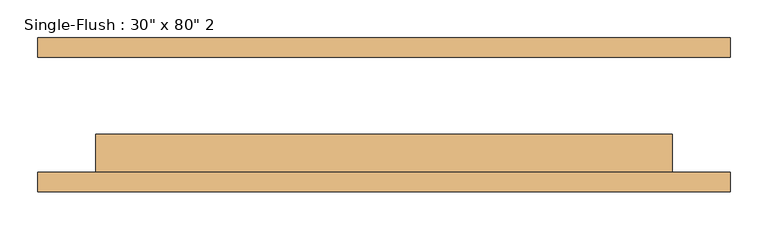
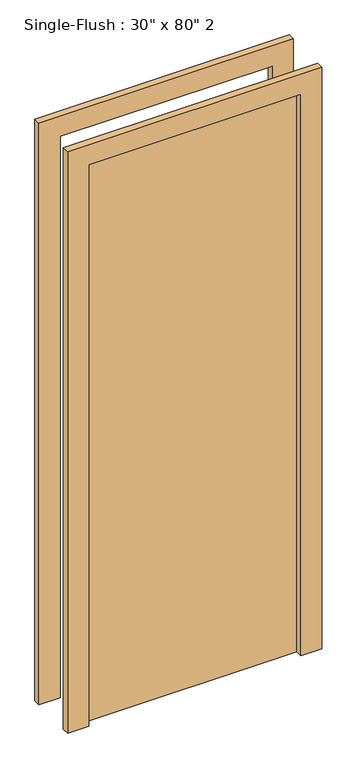
"""IFC4 building model written with IfcOpenShell, lengths in millimetres: door geometry."""

from ifc_helpers import new_model, si_unit, frame, origin, origin_with_axes, place, context, project, spatial, polyline, outline, extrude, source, transform, mapped, element, save


def door_e2b13fe9(model_context):
    return source(origin(), model_context, "Body", "SweptSolid", [
        extrude(outline(polyline([(2209.8, -457.2), (0.0, -457.2), (0.0, -381.0), (2133.6, -381.0), (2133.6, 381.0), (0.0, 381.0), (0.0, 457.2), (2209.8, 457.2), (2209.8, -457.2)])), frame((0.0, -101.6, 0.0), z_axis=(0.0, 1.0, 0.0), x_axis=(0.0, 0.0, 1.0)), (0.0, 0.0, 1.0), 25.4),
        extrude(outline(polyline([(2209.8, 457.2), (2209.8, -457.2), (0.0, -457.2), (0.0, -381.0), (2133.6, -381.0), (2133.6, 381.0), (0.0, 381.0), (0.0, 457.2), (2209.8, 457.2)])), frame((0.0, 76.2, 0.0), z_axis=(0.0, 1.0, 0.0), x_axis=(0.0, 0.0, 1.0)), (0.0, 0.0, 1.0), 25.4),
        extrude(outline(polyline([(381.0, -25.4), (381.0, -76.2), (-381.0, -76.2), (-381.0, -25.4), (381.0, -25.4)])), origin_with_axes(), (0.0, 0.0, 1.0), 2133.6),
    ])


if __name__ == "__main__":
    model = new_model("IFC4")
    model_context = context("Model", 3, world=origin())
    ifc_project = project(units=[si_unit("LENGTHUNIT", "METRE", prefix="MILLI")], contexts=[model_context])
    site = spatial("IfcSite", under=ifc_project)
    building = spatial("IfcBuilding", under=site)
    placement = place(None, origin())
    door_shape = door_e2b13fe9(model_context)
    element("IfcDoor", 1, ObjectType="Single-Flush : 30\" x 80\" 2", at=placement, inside=building, context=model_context, shape_type="MappedRepresentation", body=[
        mapped(door_shape, transform((0.0, 0.0, 0.0), x_axis=(1.0, 0.0, 0.0), y_axis=(0.0, 1.0, 0.0), z_axis=(0.0, 0.0, 1.0))),
    ])
    save(model, "model.ifc")

# Revit data of these elements
# Type "Single-Flush : 30\" x 80\" 2"
#   Type Mark = "14"
#   Construction Type Id = "MDOOR"
#   Assembly Code = "C1020"
#   Analytic Construction = "Metal"
#   Thickness = 0' - 2"
#   Heat Transfer Coefficient (U) = 0.651978 BTU/(h·ft²·°F)
#   Height = 7' - 0"
#   Trim Projection Ext = 0' - 1"
#   Trim Projection Int = 0' - 1"
#   Trim Width = 0' - 3"
#   Width = 2' - 6"
#   Define Thermal Properties by = 1
#   Door Material = Door - Panel
#   Frame Material = Door - Frame
#   Visual Light Transmittance = 0
#   Solar Heat Gain Coefficient = 0
#   Function = (empty or 0)
#   Wall Closure = (empty or 0)
# Element 1 (IfcDoor, "Single-Flush : 30\" x 80\" 2")
#   Materials on its faces: "Door - Frame", "Door - Panel"
# Materials
#   "Door - Panel": class "Wood", colour RGB 210 159 95, transparency 0, Cost = 0
#   "Door - Frame": colour RGB 118 70 51, transparency 0, Cost = 0
